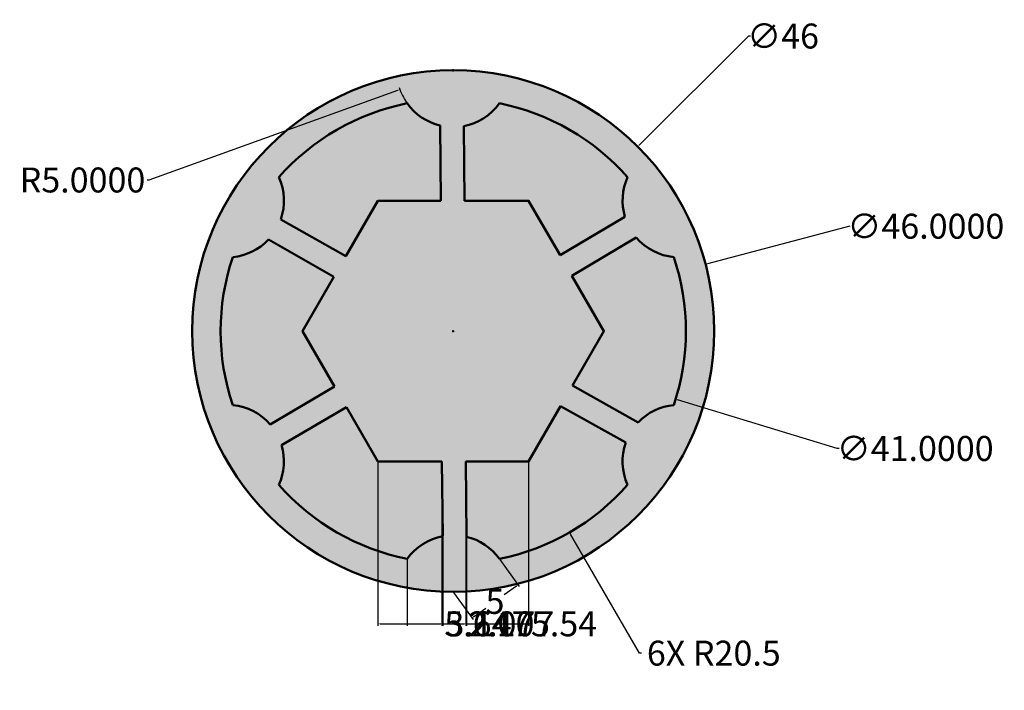
# Model space of a CAD drawing. Units: inches. Extents: x 943.1 to 1029.8, y -642.4 to -583.2.
import ezdxf

# ---------------------------------------------------------------- set-up
doc = ezdxf.new("R2010")
doc.units = ezdxf.units.IN
doc.header["$MEASUREMENT"] = 0
for name, color, linetype, lineweight in [('M-DIMS', 2, 'Continuous', 25), ('M-HATC', 252, 'Continuous', 18), ('M-OUTL', 7, 'Continuous', 50)]:
    doc.layers.add(name, color=color, linetype=linetype, lineweight=lineweight)
doc.styles.get("Standard").update_dxf_attribs({"font": 'arial.ttf'})
doc.dimstyles.get("Standard").update_dxf_attribs({"dimtxt": 2.2, "dimasz": 0.18, "dimexe": 0.18, "dimexo": 0.0625, "dimgap": 0.09, "dimtad": 0, "dimtih": 1, "dimtoh": 1, "dimdec": 4, "dimzin": 0, "dimdsep": 46, "dimtxsty": 'Standard', "dimcen": 0.09, "dimadec": 0, "dimazin": 0, "dimtfac": 1, "dimtdec": 4, "dimtofl": 0, "dimtmove": 0, "dimatfit": 3, "dimfxl": 1, "dimtolj": 1, "dimtzin": 0, "dimarcsym": 0})

# ---------------------------------------------------------------- blocks, each defined once
blk = doc.blocks.new('*U1')
for p, q in [((-1.099, -4.296), (-1.156, 2.339)), ((1, -4.296), (0.921, 2.289))]:
    blk.add_line(p, q)
for start, end in [(215.55764, 256.6264), (280.61079, 324.44236)]:
    blk.add_arc((0, 7.204), 5, start, end)
blk = doc.blocks.new('*U2')
at = {"layer": 'M-OUTL', "color": 0, "linetype": 'ByBlock', "lineweight": -2, "transparency": 16777216}
blk.add_blockref('*U1', (981.288, -594.868), dxfattribs=at)
for p, rotation in [((967.608, -602.766), 59.99999999999999), ((994.968, -602.766), 300), ((967.608, -618.562), 120), ((994.968, -618.562), 240), ((981.288, -626.46), 180)]:
    blk.add_blockref('*U1', p, dxfattribs=dict(at, rotation=rotation))
blk = doc.blocks.new('*D3')
at = {"layer": 'Defpoints', "color": 0, "transparency": 16777216}
for p in [(981.288, -587.664), (976.585, -589.362)]:
    blk.add_point(p, dxfattribs=at)
at = {"layer": 'M-DIMS', "color": 0, "lineweight": -2, "transparency": 16777216}
for p, q in [((981.198, -587.664), (981.378, -587.664)), ((981.288, -587.754), (981.288, -587.574)), ((954.504, -597.337), (976.416, -589.423)), ((954.324, -597.337), (954.504, -597.337))]:
    blk.add_line(p, q, dxfattribs=at)
blk.add_arc((981.288, -587.664), 5, 197.79396, 214.84145, dxfattribs=at)
at = {"layer": 'M-DIMS', "color": 0, "transparency": 16777216}
blk.add_solid([(976.406, -589.395), (976.426, -589.452), (976.585, -589.362)], dxfattribs=at)
at = {"layer": 'M-DIMS', "color": 0, "transparency": 16777216, "insert": (948.618, -597.337), "char_height": 2.2, "attachment_point": 5}
blk.add_mtext('\\A1;R5.0000', dxfattribs=at)
blk = doc.blocks.new('*D4')
at = {"layer": 'Defpoints', "color": 0, "transparency": 16777216}
for p in [(1003.522, -604.778), (959.054, -616.549)]:
    blk.add_point(p, dxfattribs=at)
at = {"layer": 'M-DIMS', "color": 0, "lineweight": -2, "transparency": 16777216}
for p, q in [((1016.226, -601.416), (1003.696, -604.732)), ((981.198, -610.664), (981.378, -610.664)), ((981.288, -610.754), (981.288, -610.574))]:
    blk.add_line(p, q, dxfattribs=at)
at = {"layer": 'M-DIMS', "color": 0, "transparency": 16777216}
blk.add_solid([(1003.689, -604.703), (1003.704, -604.761), (1003.522, -604.778)], dxfattribs=at)
at = {"layer": 'M-DIMS', "color": 0, "transparency": 16777216, "insert": (1022.93, -601.416), "char_height": 2.2, "attachment_point": 5}
blk.add_mtext('\\A1;∅46.0000', dxfattribs=at)
blk = doc.blocks.new('*D5')
at = {"layer": 'Defpoints', "color": 0, "transparency": 16777216}
for p in [(961.686, -604.663), (1000.89, -616.665)]:
    blk.add_point(p, dxfattribs=at)
at = {"layer": 'M-DIMS', "color": 0, "lineweight": -2, "transparency": 16777216}
for p, q in [((981.198, -610.664), (981.378, -610.664)), ((981.288, -610.754), (981.288, -610.574)), ((1015.105, -621.017), (1001.062, -616.718)), ((1015.285, -621.017), (1015.105, -621.017))]:
    blk.add_line(p, q, dxfattribs=at)
at = {"layer": 'M-DIMS', "color": 0, "transparency": 16777216}
blk.add_solid([(1001.071, -616.689), (1001.053, -616.747), (1000.89, -616.665)], dxfattribs=at)
at = {"layer": 'M-DIMS', "color": 0, "transparency": 16777216, "insert": (1021.989, -621.017), "char_height": 2.2, "attachment_point": 5}
blk.add_mtext('\\A1;∅41.0000', dxfattribs=at)
blk = doc.blocks.new('*D6')
at = {"layer": 'Defpoints', "color": 0, "transparency": 16777216}
for p in [(980.288, -622.164), (982.387, -622.164), (982.387, -636.489)]:
    blk.add_point(p, dxfattribs=at)
at = {"layer": 'M-DIMS', "color": 0, "lineweight": -2, "transparency": 16777216}
for p, q in [((980.288, -622.226), (980.288, -636.669)), ((982.387, -622.226), (982.387, -636.669)), ((980.468, -636.489), (982.207, -636.489)), ((982.387, -636.489), (982.567, -636.489))]:
    blk.add_line(p, q, dxfattribs=at)
at = {"layer": 'M-DIMS', "color": 0, "transparency": 16777216}
for points in [[(980.468, -636.459), (980.468, -636.519), (980.288, -636.489)], [(982.207, -636.459), (982.207, -636.519), (982.387, -636.489)]]:
    blk.add_solid(points, dxfattribs=at)
at = {"layer": 'M-DIMS', "color": 0, "transparency": 16777216, "insert": (985.53, -636.489), "char_height": 2.2, "attachment_point": 5}
blk.add_mtext('\\A1;2.10', dxfattribs=at)
blk = doc.blocks.new('*D7')
at = {"layer": 'Defpoints', "color": 0, "transparency": 16777216}
for p in [(974.649, -622.164), (980.288, -622.164), (980.288, -636.489)]:
    blk.add_point(p, dxfattribs=at)
at = {"layer": 'M-DIMS', "color": 0, "lineweight": -2, "transparency": 16777216}
for p, q in [((974.649, -622.226), (974.649, -636.669)), ((980.288, -622.226), (980.288, -636.669)), ((974.829, -636.489), (980.108, -636.489)), ((980.288, -636.489), (980.468, -636.489))]:
    blk.add_line(p, q, dxfattribs=at)
at = {"layer": 'M-DIMS', "color": 0, "transparency": 16777216}
for points in [[(974.829, -636.459), (974.829, -636.519), (974.649, -636.489)], [(980.108, -636.459), (980.108, -636.519), (980.288, -636.489)]]:
    blk.add_solid(points, dxfattribs=at)
at = {"layer": 'M-DIMS', "color": 0, "transparency": 16777216, "insert": (983.411, -636.489), "char_height": 2.2, "attachment_point": 5}
blk.add_mtext('\\A1;5.64', dxfattribs=at)
blk = doc.blocks.new('*D8')
at = {"layer": 'Defpoints', "color": 0, "transparency": 16777216}
for p in [(982.387, -622.164), (987.928, -622.164), (987.928, -636.489)]:
    blk.add_point(p, dxfattribs=at)
at = {"layer": 'M-DIMS', "color": 0, "lineweight": -2, "transparency": 16777216}
for p, q in [((982.387, -622.226), (982.387, -636.669)), ((987.928, -622.226), (987.928, -636.669)), ((982.567, -636.489), (987.748, -636.489)), ((987.928, -636.489), (988.108, -636.489))]:
    blk.add_line(p, q, dxfattribs=at)
at = {"layer": 'M-DIMS', "color": 0, "transparency": 16777216}
for points in [[(982.567, -636.459), (982.567, -636.519), (982.387, -636.489)], [(987.748, -636.459), (987.748, -636.519), (987.928, -636.489)]]:
    blk.add_solid(points, dxfattribs=at)
at = {"layer": 'M-DIMS', "color": 0, "transparency": 16777216, "insert": (991.05, -636.489), "char_height": 2.2, "attachment_point": 5}
blk.add_mtext('\\A1;5.54', dxfattribs=at)
blk = doc.blocks.new('*D9')
at = {"layer": 'Defpoints', "color": 0, "transparency": 16777216}
for p in [(980.367, -628.749), (982.445, -628.8), (982.445, -636.489)]:
    blk.add_point(p, dxfattribs=at)
at = {"layer": 'M-DIMS', "color": 0, "lineweight": -2, "transparency": 16777216}
for p, q in [((980.367, -628.812), (980.367, -636.669)), ((982.445, -628.862), (982.445, -636.669)), ((980.547, -636.489), (982.265, -636.489)), ((982.445, -636.489), (982.625, -636.489))]:
    blk.add_line(p, q, dxfattribs=at)
at = {"layer": 'M-DIMS', "color": 0, "transparency": 16777216}
for points in [[(980.547, -636.459), (980.547, -636.519), (980.367, -636.489)], [(982.265, -636.459), (982.265, -636.519), (982.445, -636.489)]]:
    blk.add_solid(points, dxfattribs=at)
at = {"layer": 'M-DIMS', "color": 0, "transparency": 16777216, "insert": (986.445, -636.489), "char_height": 2.2, "attachment_point": 5}
blk.add_mtext('\\A1;2.077', dxfattribs=at)
blk = doc.blocks.new('*D10')
at = {"layer": 'Defpoints', "color": 0, "transparency": 16777216}
for p in [(980.367, -628.749), (977.22, -630.756), (980.367, -636.489)]:
    blk.add_point(p, dxfattribs=at)
at = {"layer": 'M-DIMS', "color": 0, "lineweight": -2, "transparency": 16777216}
for p, q in [((980.367, -628.812), (980.367, -636.669)), ((977.22, -630.819), (977.22, -636.669)), ((977.4, -636.489), (980.187, -636.489)), ((980.367, -636.489), (980.547, -636.489))]:
    blk.add_line(p, q, dxfattribs=at)
at = {"layer": 'M-DIMS', "color": 0, "transparency": 16777216}
for points in [[(977.4, -636.459), (977.4, -636.519), (977.22, -636.489)], [(980.187, -636.459), (980.187, -636.519), (980.367, -636.489)]]:
    blk.add_solid(points, dxfattribs=at)
at = {"layer": 'M-DIMS', "color": 0, "transparency": 16777216, "insert": (984.349, -636.489), "char_height": 2.2, "attachment_point": 5}
blk.add_mtext('\\A1;3.147', dxfattribs=at)
blk = doc.blocks.new('*D11')
at = {"layer": 'Defpoints', "color": 0, "transparency": 16777216}
for p in [(985.356, -630.756), (981.288, -633.664), (982.931, -635.962)]:
    blk.add_point(p, dxfattribs=at)
at = {"layer": 'M-DIMS', "color": 0, "lineweight": -2, "transparency": 16777216}
for p, q in [((985.392, -630.807), (987.103, -633.201)), ((986.852, -633.159), (985.784, -633.923)), ((981.324, -633.715), (983.036, -636.109)), ((983.077, -635.857), (984.145, -635.094))]:
    blk.add_line(p, q, dxfattribs=at)
at = {"layer": 'M-DIMS', "color": 0, "transparency": 16777216}
for points in [[(986.835, -633.135), (986.87, -633.184), (986.999, -633.055)], [(983.06, -635.833), (983.095, -635.882), (982.931, -635.962)]]:
    blk.add_solid(points, dxfattribs=at)
at = {"layer": 'M-DIMS', "color": 0, "transparency": 16777216, "insert": (984.965, -634.508), "char_height": 2.2, "attachment_point": 5}
blk.add_mtext('\\A1;5', dxfattribs=at)
blk = doc.blocks.new('*D12')
at = {"layer": 'Defpoints', "color": 0, "transparency": 16777216}
for p in [(997.551, -594.399), (965.026, -626.928)]:
    blk.add_point(p, dxfattribs=at)
at = {"layer": 'M-DIMS', "color": 0, "lineweight": -2, "transparency": 16777216}
for p, q in [((1007.308, -584.641), (997.678, -594.272)), ((1007.488, -584.641), (1007.308, -584.641)), ((981.198, -610.664), (981.378, -610.664)), ((981.288, -610.754), (981.288, -610.574))]:
    blk.add_line(p, q, dxfattribs=at)
at = {"layer": 'M-DIMS', "color": 0, "transparency": 16777216}
blk.add_solid([(997.657, -594.251), (997.699, -594.293), (997.551, -594.399)], dxfattribs=at)
at = {"layer": 'M-DIMS', "color": 0, "transparency": 16777216, "insert": (1010.35, -584.641), "char_height": 2.2, "attachment_point": 5}
blk.add_mtext('\\A1;∅46', dxfattribs=at)
blk = doc.blocks.new('*D13')
at = {"layer": 'Defpoints', "color": 0, "transparency": 16777216}
for p in [(981.288, -610.664), (991.538, -628.417)]:
    blk.add_point(p, dxfattribs=at)
at = {"layer": 'M-DIMS', "color": 0, "lineweight": -2, "transparency": 16777216}
for p, q in [((981.198, -610.664), (981.378, -610.664)), ((981.288, -610.754), (981.288, -610.574)), ((997.688, -639.069), (991.628, -628.573)), ((997.868, -639.069), (997.688, -639.069))]:
    blk.add_line(p, q, dxfattribs=at)
at = {"layer": 'M-DIMS', "color": 0, "transparency": 16777216}
blk.add_solid([(991.654, -628.558), (991.602, -628.588), (991.538, -628.417)], dxfattribs=at)
at = {"layer": 'M-DIMS', "color": 0, "transparency": 16777216, "insert": (1004.246, -639.069), "char_height": 2.2, "attachment_point": 5}
blk.add_mtext('\\A1;6X R20.5', dxfattribs=at)

msp = doc.modelspace()

# ---------------------------------------------------------------- hatches: boundary and pattern name
at = {"layer": 'M-HATC'}
h = msp.add_hatch(color=256, dxfattribs=at)
h.dxf.hatch_style = 1
h.paths.add_polyline_path([(958.28812, -610.66394, 1), (1004.28812, -610.66394, 1)])
h.paths.add_polyline_path([(980.13162, -592.52835), (980.18888, -599.16394), (974.64859, -599.16394), (971.82883, -604.04791), (966.08596, -600.82386, 0.1936177), (965.92143, -597.09505, -0.16335571), (977.22047, -590.57155, 0.18113929)], flags=16)
h.paths.add_polyline_path([(982.2088, -592.57844, 0.1936177), (985.35577, -590.57155, -0.16335571), (996.65481, -597.09505, 0.18113929), (996.41575, -600.59459), (990.69779, -603.96197), (987.92765, -599.16394), (982.28812, -599.16394)], flags=16)
h.paths.add_polyline_path([(970.77921, -605.86591), (968.00906, -610.66394), (970.82883, -615.54791), (965.16528, -618.90935, 0.1936177), (961.85377, -617.18744, -0.16335571), (961.85377, -604.14044, 0.18113929), (965.00399, -602.5977)], flags=16)
h.paths.add_polyline_path([(991.74741, -605.77997), (997.41096, -602.41853, 0.1936177), (1000.72247, -604.14044, -0.16335571), (1000.72247, -617.18744, 0.18113929), (997.57225, -618.73018), (991.79703, -615.46197), (994.56718, -610.66394)], flags=16)
h.paths.add_polyline_path([(971.87845, -617.36591), (974.64859, -622.16394), (980.28812, -622.16394), (980.36744, -628.74944, 0.1936177), (977.22047, -630.75633, -0.16335571), (965.92143, -624.23283, 0.18113929), (966.16049, -620.73329)], flags=16)
h.paths.add_polyline_path([(990.74741, -617.27997), (996.49028, -620.50402, 0.1936177), (996.65481, -624.23283, -0.16335571), (985.35577, -630.75633, 0.18113929), (982.44462, -628.79953), (982.38736, -622.16394), (987.92765, -622.16394)], flags=16)
h = msp.add_hatch(color=256, dxfattribs=at)
h.dxf.hatch_style = 1
h.paths.add_polyline_path([(985.35577, -590.57155, -0.1936177), (982.2088, -592.57844), (982.28812, -599.16394), (987.92765, -599.16394), (990.69779, -603.96197), (996.41575, -600.59459, -0.18113929), (996.65481, -597.09505, 0.16335571)])
h.paths.add_polyline_path([(980.13162, -592.52835, -0.18113929), (977.22047, -590.57155, 0.16335571), (965.92143, -597.09505, -0.1936177), (966.08596, -600.82386), (971.82883, -604.04791), (974.64859, -599.16394), (980.18888, -599.16394)])
h.paths.add_polyline_path([(970.77921, -605.86591), (965.00399, -602.5977, -0.18113929), (961.85377, -604.14044, 0.16335571), (961.85377, -617.18744, -0.1936177), (965.16528, -618.90935), (970.82883, -615.54791), (968.00906, -610.66394)])
h.paths.add_polyline_path([(971.87845, -617.36591), (966.16049, -620.73329, -0.18113929), (965.92143, -624.23283, 0.16335571), (977.22047, -630.75633, -0.1936177), (980.36744, -628.74944), (980.28812, -622.16394), (974.64859, -622.16394)])
h.paths.add_polyline_path([(996.49028, -620.50402), (990.74741, -617.27997), (987.92765, -622.16394), (982.38736, -622.16394), (982.44462, -628.79953, -0.18113929), (985.35577, -630.75633, 0.16335571), (996.65481, -624.23283, -0.1936177)])
h.paths.add_polyline_path([(1000.72247, -604.14044, -0.1936177), (997.41096, -602.41853), (991.74741, -605.77997), (994.56718, -610.66394), (991.79703, -615.46197), (997.57225, -618.73018, -0.18113929), (1000.72247, -617.18744, 0.16335571)])

# ---------------------------------------------------------------- linework, layer by layer
at = {"layer": 'M-OUTL'}
for points in [[(980.18888, -599.16394), (974.64859, -599.16394), (971.82883, -604.04791)], [(990.69779, -603.96197), (987.92765, -599.16394), (982.28812, -599.16394)], [(970.77921, -605.86591), (968.00906, -610.66394), (970.82883, -615.54791)], [(991.79703, -615.46197), (994.56718, -610.66394), (991.74741, -605.77997)], [(971.87845, -617.36591), (974.64859, -622.16394), (980.28812, -622.16394)], [(982.38736, -622.16394), (987.92765, -622.16394), (990.74741, -617.27997)]]:
    msp.add_lwpolyline(points, dxfattribs=at)
msp.add_circle((981.28812, -610.66394), 23, dxfattribs=at)
for start, end in [(101.4447065, 138.5552935), (41.4447065, 78.5552935), (161.4447065, 198.5552935), (341.4447065, 18.5552935), (221.4447065, 258.5552935), (281.4447065, 318.5552935)]:
    msp.add_arc((981.28812, -610.66394), 20.5, start, end, dxfattribs=at)

# ---------------------------------------------------------------- block references
msp.add_blockref('*U2', (0, 0), dxfattribs=at)

# ---------------------------------------------------------------- dimensions: what is measured, and where the dimension line sits
at = {"layer": 'M-DIMS'}
for p1, p2, override, picture, middle in [((965.02569, -626.92843), (997.55055, -594.39945), {"dimdec": 0, "dimlfac": 1, "dimrnd": 0, "dimzin": 0, "dimdsep": 46, "dimlunit": 2}, '*D12', (1010.34976, -584.64076)), ((959.0539, -616.54948), (1003.52234, -604.7784), {"dimclrd": 0, "dimclre": 0, "dimclrt": 0}, '*D4', (1016.22589, -601.4157)), ((961.68623, -604.6626), (1000.89001, -616.66528), {"dimclrd": 0, "dimclre": 0, "dimclrt": 0}, '*D5', (1021.98909, -621.01731))]:
    dim = msp.add_diameter_dim_2p(p1=p1, p2=p2, dimstyle='Standard', override=override, dxfattribs=at)
    dim.commit()
    dim.dimension.update_dxf_attribs({"geometry": picture, "text_midpoint": middle, "dimtype": 163})
dim = msp.add_radius_dim(center=(981.28812, -587.66394), mpoint=(976.58539, -589.36228), dimstyle='Standard', override={"dimclrd": 0, "dimclre": 0, "dimclrt": 0}, dxfattribs=at)
dim.commit()
dim.dimension.update_dxf_attribs({"geometry": '*D3', "text_midpoint": (948.61818, -597.33682), "dimtype": 164})
dim = msp.add_radius_dim(center=(981.28812, -610.66394), mpoint=(991.53823, -628.4174), text='6X <>', dimstyle='Standard', override={"dimdec": 1, "dimlfac": 1, "dimrnd": 0, "dimzin": 0, "dimdsep": 46, "dimlunit": 2}, dxfattribs=at)
dim.commit()
dim.dimension.update_dxf_attribs({"geometry": '*D13', "text_midpoint": (1004.24615, -639.06947), "dimtype": 164})
for base, p1, p2, override, picture, middle in [((980.28812, -636.48894), (974.64859, -622.16394), (980.28812, -622.16394), {"dimdec": 2, "dimlfac": 1, "dimrnd": 0, "dimzin": 0, "dimdsep": 46, "dimlunit": 2}, '*D7', (983.41092, -636.48894)), ((982.38736, -636.48894), (980.28812, -622.16394), (982.38736, -622.16394), {"dimdec": 2, "dimlfac": 1, "dimrnd": 0, "dimzin": 0, "dimdsep": 46, "dimlunit": 2}, '*D6', (985.52966, -636.48894)), ((987.92765, -636.48894), (982.38736, -622.16394), (987.92765, -622.16394), {"dimdec": 2, "dimlfac": 1, "dimrnd": 0, "dimzin": 0, "dimdsep": 46, "dimlunit": 2}, '*D8', (991.05045, -636.48894)), ((980.36744, -636.48894), (977.22047, -630.75633), (980.36744, -628.74944), {"dimdec": 3, "dimlfac": 1, "dimrnd": 0, "dimzin": 0, "dimdsep": 46, "dimlunit": 2}, '*D10', (984.34862, -636.48894)), ((982.44462, -636.48894), (980.36744, -628.74944), (982.44462, -628.79953), {"dimdec": 3, "dimlfac": 1, "dimrnd": 0, "dimzin": 0, "dimdsep": 46, "dimlunit": 2}, '*D9', (986.44531, -636.48894))]:
    dim = msp.add_linear_dim(base=base, p1=p1, p2=p2, dimstyle='Standard', override=override, dxfattribs=at)
    dim.commit()
    dim.dimension.update_dxf_attribs({"geometry": picture, "text_midpoint": middle})
dim = msp.add_linear_dim(base=(982.93092, -635.96216), p1=(985.35577, -630.75633), p2=(981.28812, -633.66394), angle=215.557645, dimstyle='Standard', override={"dimdec": 0, "dimlfac": 1, "dimrnd": 0, "dimzin": 0, "dimdsep": 46, "dimlunit": 2}, dxfattribs=at)
dim.commit()
dim.dimension.update_dxf_attribs({"geometry": '*D11', "text_midpoint": (984.96475, -634.50836)})

doc.saveas('drawing.dxf')
